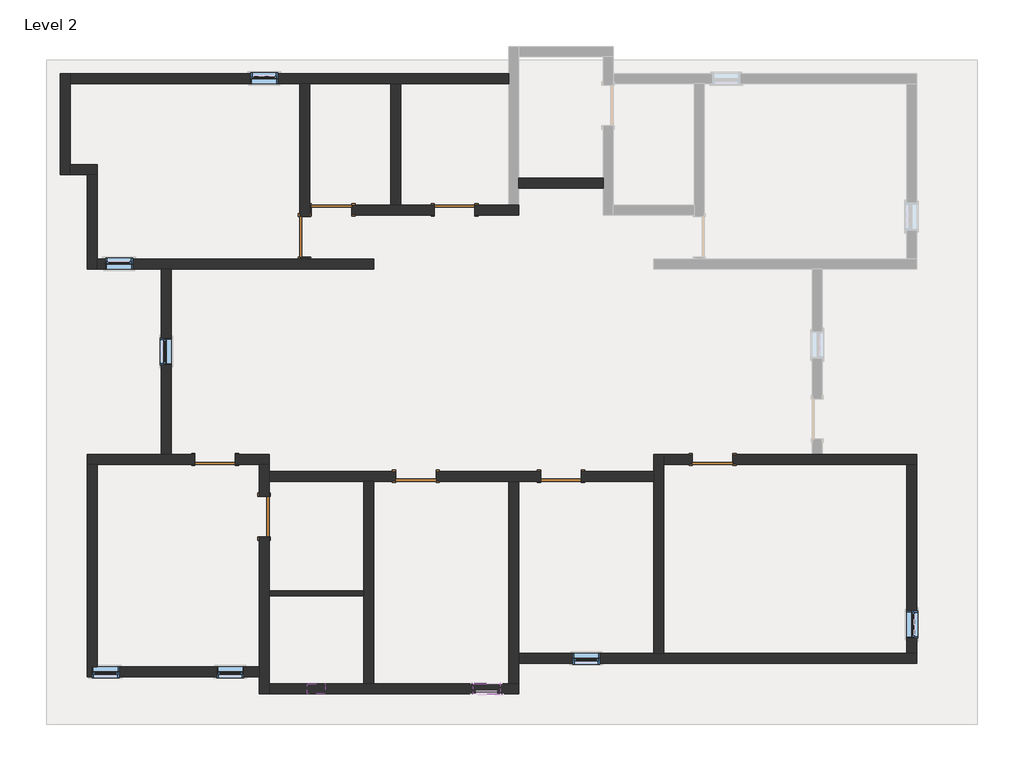
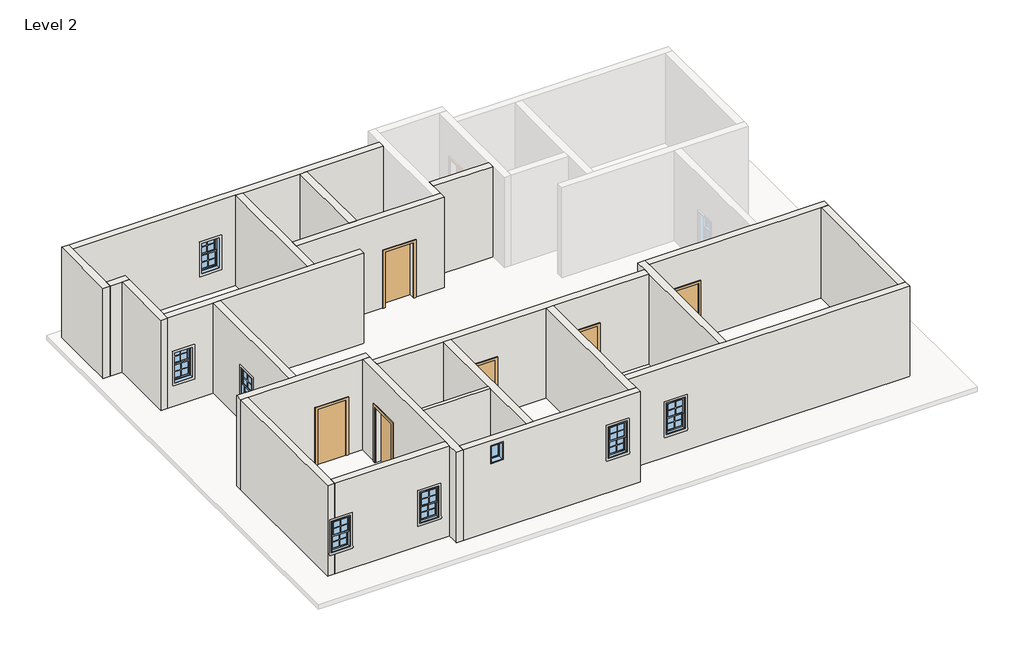
# One storey, part 1 of 2: 23 walls, 9 windows, 8 doors.
"""IFC4 building model written with IfcOpenShell, lengths in millimetres."""

from ifc_helpers import new_model, si_unit, frame, origin, place, context, project, spatial, polyline, outline, extrude, faceted_brep, transform, mapped, element, save
from components import door_89fc3733, door_ef0d591a, window_aa618e30, window_d92165b9

model = new_model("IFC4")

# Units and contexts
model_context = context("Model", 3, world=origin())
ifc_project = project(units=[si_unit("LENGTHUNIT", "METRE", prefix="MILLI")], contexts=[model_context])

# Site, building, storey
site = spatial("IfcSite", under=ifc_project)
building = spatial("IfcBuilding", under=site)
storey = spatial("IfcBuildingStorey", under=building, Name="Level 2", Elevation=3200.4)

# Doors
placement = place(None, origin())
door_shape = door_89fc3733(model_context)
element("IfcDoor", 1, ObjectType="Single-Flush : 36\" x 80\"", at=placement, inside=storey, context=model_context, shape_type="MappedRepresentation", body=[
    mapped(door_shape, transform((-6055.8415084, -1138.2064015, 3200.4), x_axis=(-1.0, 0.0, 0.0), y_axis=(0.0, -1.0, 0.0), z_axis=(0.0, 0.0, 1.0))),
])
element("IfcDoor", 2, ObjectType="Single-Flush : 36\" x 80\"", at=placement, inside=storey, context=model_context, shape_type="MappedRepresentation", body=[
    mapped(door_shape, transform((649.7584916, -757.2064015, 3200.4), x_axis=(-1.0, 0.0, 0.0), y_axis=(0.0, -1.0, 0.0), z_axis=(0.0, 0.0, 1.0))),
])
element("IfcDoor", 3, ObjectType="Single-Flush : 36\" x 80\"", at=placement, inside=storey, context=model_context, shape_type="MappedRepresentation", body=[
    mapped(door_shape, transform((-5179.5415084, 4881.5935985, 3200.4), x_axis=(1.0, 0.0, 0.0), y_axis=(0.0, 1.0, 0.0), z_axis=(0.0, 0.0, 1.0))),
])
element("IfcDoor", 4, ObjectType="Single-Flush : 36\" x 80\"", at=placement, inside=storey, context=model_context, shape_type="MappedRepresentation", body=[
    mapped(door_shape, transform((-2779.2415084, -1138.2064015, 3200.4), x_axis=(-1.0, 0.0, 0.0), y_axis=(0.0, -1.0, 0.0), z_axis=(0.0, 0.0, 1.0))),
])
door_2_shape = door_ef0d591a(model_context)
element("IfcDoor", 5, ObjectType="Single-Flush : 36\" x 80\"", at=placement, inside=storey, context=model_context, shape_type="MappedRepresentation", body=[
    mapped(door_2_shape, transform((-8570.4415084, 4271.9935985, 3200.4), x_axis=(0.0, -1.0, 0.0), y_axis=(1.0, 0.0, 0.0), z_axis=(0.0, 0.0, 1.0))),
])
element("IfcDoor", 6, ObjectType="Single-Flush : 36\" x 80\"", at=placement, inside=storey, context=model_context, shape_type="MappedRepresentation", body=[
    mapped(door_2_shape, transform((-7960.8415084, 4881.5935985, 3200.4), x_axis=(-1.0, 0.0, 0.0), y_axis=(0.0, -1.0, 0.0), z_axis=(0.0, 0.0, 1.0))),
])
element("IfcDoor", 7, ObjectType="Single-Flush : 36\" x 80\"", at=placement, inside=storey, context=model_context, shape_type="MappedRepresentation", body=[
    mapped(door_2_shape, transform((-9484.8415084, -2052.6064015, 3200.4), x_axis=(0.0, 1.0, 0.0), y_axis=(-1.0, 0.0, 0.0), z_axis=(0.0, 0.0, 1.0))),
])
element("IfcDoor", 8, ObjectType="Single-Flush : 36\" x 80\"", at=placement, inside=storey, context=model_context, shape_type="MappedRepresentation", body=[
    mapped(door_2_shape, transform((-10589.7415084, -757.2064015, 3200.4), x_axis=(1.0, 0.0, 0.0), y_axis=(0.0, 1.0, 0.0), z_axis=(0.0, 0.0, 1.0))),
])

# Walls
element("IfcWall", 9, ObjectType="4.5\"", at=placement, inside=storey, context=model_context, shape_type="SweptSolid", body=[
    extrude(outline(polyline([(-7236.9415084, -3843.3848078), (-9370.5415084, -3843.3848078), (-9370.5415084, -3729.0848078), (-7236.9415084, -3729.0848078), (-7236.9415084, -3843.3848078)])), frame((0.0, 0.0, 3200.4), z_axis=(0.0, 0.0, 1.0), x_axis=(1.0, 0.0, 0.0)), (0.0, 0.0, 1.0), 3200.4),
])
element("IfcWall", 10, ObjectType="9\"", at=placement, inside=storey, context=model_context, shape_type="Brep", body=[
    faceted_brep([(-14094.9415084, 7967.6935985, 3200.4), (-14094.9415084, 5681.6935985, 3200.4), (-14094.9415084, 5681.6935985, 6400.8), (-14094.9415084, 7967.6935985, 6400.8), (-13866.3415084, 7967.6935985, 3200.4), (-13866.3415084, 7967.6935985, 6400.8), (-13866.3415084, 7739.0935985, 6400.8), (-13866.3415084, 5910.2935985, 6400.8), (-13866.3415084, 5681.6935985, 6400.8), (-13866.3415084, 5681.6935985, 3200.4), (-13866.3415084, 5910.2935985, 3200.4), (-13866.3415084, 7739.0935985, 3200.4)], [[[0, 1, 2, 3]], [[4, 5, 6, 7, 8, 9, 10, 11]], [[1, 0, 4, 11, 10, 9]], [[3, 2, 8, 7, 6, 5]], [[2, 1, 9, 8]], [[0, 3, 5, 4]]]),
])
element("IfcWall", 11, ObjectType="9\"", at=placement, inside=storey, context=model_context, shape_type="Brep", body=[
    faceted_brep([(-13866.3415084, 5681.6935985, 3200.4), (-13485.3415084, 5681.6935985, 3200.4), (-13256.7415084, 5681.6935985, 3200.4), (-13256.7415084, 5681.6935985, 6400.8), (-13485.3415084, 5681.6935985, 6400.8), (-13866.3415084, 5681.6935985, 6400.8), (-13866.3415084, 5910.2935985, 3200.4), (-13866.3415084, 5910.2935985, 6400.8), (-13256.7415084, 5910.2935985, 6400.8), (-13256.7415084, 5910.2935985, 3200.4)], [[[0, 1, 2, 3, 4, 5]], [[6, 7, 8, 9]], [[2, 1, 0, 6, 9]], [[5, 4, 3, 8, 7]], [[0, 5, 7, 6]], [[3, 2, 9, 8]]]),
])
element("IfcWall", 12, ObjectType="9\"", at=placement, inside=storey, context=model_context, shape_type="Brep", body=[
    faceted_brep([(-13485.3415084, 5681.6935985, 3200.4), (-13485.3415084, 3548.0935985, 3200.4), (-13485.3415084, 3548.0935985, 6400.8), (-13485.3415084, 5681.6935985, 6400.8), (-13256.7415084, 5681.6935985, 3200.4), (-13256.7415084, 5681.6935985, 6400.8), (-13256.7415084, 3776.6935985, 6400.8), (-13256.7415084, 3548.0935985, 6400.8), (-13256.7415084, 3548.0935985, 3200.4), (-13256.7415084, 3776.6935985, 3200.4)], [[[0, 1, 2, 3]], [[4, 5, 6, 7, 8, 9]], [[1, 0, 4, 9, 8]], [[3, 2, 7, 6, 5]], [[0, 3, 5, 4]], [[2, 1, 8, 7]]]),
])
element("IfcWall", 13, ObjectType="9\"", at=placement, inside=storey, context=model_context, shape_type="Brep", body=[
    faceted_brep([(-13256.7415084, 3548.0935985, 3200.4), (-11808.9415084, 3548.0935985, 3200.4), (-11580.3415084, 3548.0935985, 3200.4), (-7008.3415084, 3548.0935985, 3200.4), (-7008.3415084, 3548.0935985, 6400.8), (-11580.3415084, 3548.0935985, 6400.8), (-11808.9415084, 3548.0935985, 6400.8), (-13256.7415084, 3548.0935985, 6400.8), (-13066.2415084, 3548.0935985, 5181.6), (-12456.6415084, 3548.0935985, 5181.6), (-12456.6415084, 3548.0935985, 4114.8), (-13066.2415084, 3548.0935985, 4114.8), (-13256.7415084, 3776.6935985, 3200.4), (-13256.7415084, 3776.6935985, 6400.8), (-8684.7415084, 3776.6935985, 6400.8), (-8456.1415084, 3776.6935985, 6400.8), (-7008.3415084, 3776.6935985, 6400.8), (-7008.3415084, 3776.6935985, 3200.4), (-8456.1415084, 3776.6935985, 3200.4), (-8684.7415084, 3776.6935985, 3200.4), (-13066.2415084, 3776.6935985, 5181.6), (-13066.2415084, 3776.6935985, 4114.8), (-12456.6415084, 3776.6935985, 4114.8), (-12456.6415084, 3776.6935985, 5181.6)], [[[0, 1, 2, 3, 4, 5, 6, 7], [8, 9, 10, 11]], [[12, 13, 14, 15, 16, 17, 18, 19], [20, 21, 22, 23]], [[3, 2, 1, 0, 12, 19, 18, 17]], [[4, 3, 17, 16]], [[7, 6, 5, 4, 16, 15, 14, 13]], [[0, 7, 13, 12]], [[21, 20, 8, 11]], [[22, 21, 11, 10]], [[23, 22, 10, 9]], [[20, 23, 9, 8]]]),
])
element("IfcWall", 14, ObjectType="9\"", at=placement, inside=storey, context=model_context, shape_type="Brep", body=[
    faceted_brep([(-8684.7415084, 3814.7935985, 5232.4), (-8684.7415084, 3814.7935985, 3200.4), (-8684.7415084, 3776.6935985, 3200.4), (-8684.7415084, 3776.6935985, 6400.8), (-8684.7415084, 7739.0935985, 6400.8), (-8684.7415084, 7739.0935985, 3200.4), (-8684.7415084, 4729.1935985, 3200.4), (-8684.7415084, 4729.1935985, 5232.4), (-8456.1415084, 3776.6935985, 3200.4), (-8456.1415084, 3814.7935985, 3200.4), (-8456.1415084, 3814.7935985, 5232.4), (-8456.1415084, 4729.1935985, 5232.4), (-8456.1415084, 4729.1935985, 3200.4), (-8456.1415084, 4767.2935985, 3200.4), (-8456.1415084, 4995.8935985, 3200.4), (-8456.1415084, 7739.0935985, 3200.4), (-8456.1415084, 7739.0935985, 6400.8), (-8456.1415084, 4995.8935985, 6400.8), (-8456.1415084, 4767.2935985, 6400.8), (-8456.1415084, 3776.6935985, 6400.8)], [[[0, 1, 2, 3, 4, 5, 6, 7]], [[8, 9, 10, 11, 12, 13, 14, 15, 16, 17, 18, 19]], [[6, 5, 15, 14, 13, 12]], [[2, 1, 9, 8]], [[4, 3, 19, 18, 17, 16]], [[3, 2, 8, 19]], [[5, 4, 16, 15]], [[10, 9, 1, 0]], [[11, 10, 0, 7]], [[12, 11, 7, 6]]]),
])
element("IfcWall", 15, ObjectType="9\"", at=placement, inside=storey, context=model_context, shape_type="Brep", body=[
    faceted_brep([(-3960.3415084, 7967.6935985, 3200.4), (-13866.3415084, 7967.6935985, 3200.4), (-13866.3415084, 7967.6935985, 6400.8), (-3960.3415084, 7967.6935985, 6400.8), (-9789.6415084, 7967.6935985, 5181.6), (-9789.6415084, 7967.6935985, 4114.8), (-9180.0415084, 7967.6935985, 4114.8), (-9180.0415084, 7967.6935985, 5181.6), (-3960.3415084, 7739.0935985, 3200.4), (-3960.3415084, 7739.0935985, 6400.8), (-6398.7415084, 7739.0935985, 6400.8), (-6627.3415084, 7739.0935985, 6400.8), (-8456.1415084, 7739.0935985, 6400.8), (-8684.7415084, 7739.0935985, 6400.8), (-13866.3415084, 7739.0935985, 6400.8), (-13866.3415084, 7739.0935985, 3200.4), (-8684.7415084, 7739.0935985, 3200.4), (-8456.1415084, 7739.0935985, 3200.4), (-6627.3415084, 7739.0935985, 3200.4), (-6398.7415084, 7739.0935985, 3200.4), (-9789.6415084, 7739.0935985, 5181.6), (-9180.0415084, 7739.0935985, 5181.6), (-9180.0415084, 7739.0935985, 4114.8), (-9789.6415084, 7739.0935985, 4114.8)], [[[0, 1, 2, 3], [4, 5, 6, 7]], [[8, 9, 10, 11, 12, 13, 14, 15, 16, 17, 18, 19], [20, 21, 22, 23]], [[1, 0, 8, 19, 18, 17, 16, 15]], [[3, 2, 14, 13, 12, 11, 10, 9]], [[2, 1, 15, 14]], [[0, 3, 9, 8]], [[5, 4, 20, 23]], [[6, 5, 23, 22]], [[7, 6, 22, 21]], [[4, 7, 21, 20]]]),
])
element("IfcWall", 16, ObjectType="9\"", at=placement, inside=storey, context=model_context, shape_type="Brep", body=[
    faceted_brep([(-3731.7415084, 4995.8935985, 3200.4), (-3960.3415084, 4995.8935985, 3200.4), (-4722.3415084, 4995.8935985, 3200.4), (-4722.3415084, 4995.8935985, 5232.4), (-5636.7415084, 4995.8935985, 5232.4), (-5636.7415084, 4995.8935985, 3200.4), (-6398.7415084, 4995.8935985, 3200.4), (-6627.3415084, 4995.8935985, 3200.4), (-7503.6415084, 4995.8935985, 3200.4), (-7503.6415084, 4995.8935985, 5232.4), (-8418.0415084, 4995.8935985, 5232.4), (-8418.0415084, 4995.8935985, 3200.4), (-8456.1415084, 4995.8935985, 3200.4), (-8456.1415084, 4995.8935985, 6400.8), (-6627.3415084, 4995.8935985, 6400.8), (-6398.7415084, 4995.8935985, 6400.8), (-3960.3415084, 4995.8935985, 6400.8), (-3731.7415084, 4995.8935985, 6400.8), (-4722.3415084, 4767.2935985, 5232.4), (-4722.3415084, 4767.2935985, 3200.4), (-3731.7415084, 4767.2935985, 3200.4), (-3731.7415084, 4767.2935985, 6400.8), (-8456.1415084, 4767.2935985, 6400.8), (-8456.1415084, 4767.2935985, 3200.4), (-8418.0415084, 4767.2935985, 3200.4), (-8418.0415084, 4767.2935985, 5232.4), (-7503.6415084, 4767.2935985, 5232.4), (-7503.6415084, 4767.2935985, 3200.4), (-5636.7415084, 4767.2935985, 3200.4), (-5636.7415084, 4767.2935985, 5232.4)], [[[0, 1, 2, 3, 4, 5, 6, 7, 8, 9, 10, 11, 12, 13, 14, 15, 16, 17]], [[18, 19, 20, 21, 22, 23, 24, 25, 26, 27, 28, 29]], [[12, 11, 24, 23]], [[28, 27, 8, 7, 6, 5]], [[20, 19, 2, 1, 0]], [[17, 16, 15, 14, 13, 22, 21]], [[13, 12, 23, 22]], [[0, 17, 21, 20]], [[25, 24, 11, 10]], [[26, 25, 10, 9]], [[27, 26, 9, 8]], [[3, 2, 19, 18]], [[4, 3, 18, 29]], [[5, 4, 29, 28]]]),
])
element("IfcWall", 17, ObjectType="9\"", at=placement, inside=storey, context=model_context, shape_type="SweptSolid", body=[
    extrude(outline(polyline([(-6627.3415084, 4995.8935985), (-6627.3415084, 7739.0935985), (-6398.7415084, 7739.0935985), (-6398.7415084, 4995.8935985), (-6627.3415084, 4995.8935985)])), frame((0.0, 0.0, 3200.4), z_axis=(0.0, 0.0, 1.0), x_axis=(1.0, 0.0, 0.0)), (0.0, 0.0, 1.0), 3200.4),
])
element("IfcWall", 18, ObjectType="9\"", at=placement, inside=storey, context=model_context, shape_type="SweptSolid", body=[
    extrude(outline(polyline([(-3731.7415084, 5605.4935985), (-1826.7415084, 5605.4935985), (-1826.7415084, 5376.8935985), (-3731.7415084, 5376.8935985), (-3731.7415084, 5605.4935985)])), frame((0.0, 0.0, 3200.4), z_axis=(0.0, 0.0, 1.0), x_axis=(1.0, 0.0, 0.0)), (0.0, 0.0, 1.0), 3200.4),
])
element("IfcWall", 19, ObjectType="9\"", at=placement, inside=storey, context=model_context, shape_type="SweptSolid", body=[
    extrude(outline(polyline([(3548.0935985, 3200.4), (-642.9064015, 3200.4), (-642.9064015, 6400.8), (3548.0935985, 6400.8), (3548.0935985, 3200.4)]), holes=[polyline([(1376.3935985, 5181.6), (1376.3935985, 4114.8), (1985.9935985, 4114.8), (1985.9935985, 5181.6), (1376.3935985, 5181.6)])]), frame((-11808.9415084, 0.0, 0.0), z_axis=(1.0, 0.0, 0.0), x_axis=(0.0, 1.0, 0.0)), (0.0, 0.0, 1.0), 228.6),
])
element("IfcWall", 20, ObjectType="9\"", at=placement, inside=storey, context=model_context, shape_type="Brep", body=[
    faceted_brep([(-9370.5415084, -642.9064015, 3200.4), (-10132.5415084, -642.9064015, 3200.4), (-10132.5415084, -642.9064015, 5232.4), (-11046.9415084, -642.9064015, 5232.4), (-11046.9415084, -642.9064015, 3200.4), (-11580.3415084, -642.9064015, 3200.4), (-11808.9415084, -642.9064015, 3200.4), (-13485.3415084, -642.9064015, 3200.4), (-13485.3415084, -642.9064015, 6400.8), (-11808.9415084, -642.9064015, 6400.8), (-11580.3415084, -642.9064015, 6400.8), (-9370.5415084, -642.9064015, 6400.8), (-10132.5415084, -871.5064015, 5232.4), (-10132.5415084, -871.5064015, 3200.4), (-9599.1415084, -871.5064015, 3200.4), (-9370.5415084, -871.5064015, 3200.4), (-9370.5415084, -871.5064015, 6400.8), (-9599.1415084, -871.5064015, 6400.8), (-13256.7415084, -871.5064015, 6400.8), (-13485.3415084, -871.5064015, 6400.8), (-13485.3415084, -871.5064015, 3200.4), (-13256.7415084, -871.5064015, 3200.4), (-11046.9415084, -871.5064015, 3200.4), (-11046.9415084, -871.5064015, 5232.4)], [[[0, 1, 2, 3, 4, 5, 6, 7, 8, 9, 10, 11]], [[12, 13, 14, 15, 16, 17, 18, 19, 20, 21, 22, 23]], [[15, 14, 13, 1, 0]], [[22, 21, 20, 7, 6, 5, 4]], [[11, 10, 9, 8, 19, 18, 17, 16]], [[8, 7, 20, 19]], [[0, 11, 16, 15]], [[2, 1, 13, 12]], [[3, 2, 12, 23]], [[4, 3, 23, 22]]]),
])
element("IfcWall", 21, ObjectType="9\"", at=placement, inside=storey, context=model_context, shape_type="Brep", body=[
    faceted_brep([(-13485.3415084, -871.5064015, 3200.4), (-13485.3415084, -5672.1064015, 3200.4), (-13485.3415084, -5672.1064015, 6400.8), (-13485.3415084, -871.5064015, 6400.8), (-13256.7415084, -5672.1064015, 3200.4), (-13256.7415084, -5443.5064015, 3200.4), (-13256.7415084, -871.5064015, 3200.4), (-13256.7415084, -871.5064015, 6400.8), (-13256.7415084, -5443.5064015, 6400.8), (-13256.7415084, -5672.1064015, 6400.8), (-13256.7415084, -5672.1064015, 5181.6), (-13256.7415084, -5443.5064015, 5181.6), (-13256.7415084, -5443.5064015, 4114.8), (-13256.7415084, -5672.1064015, 4114.8), (-13371.0415084, -5672.1064015, 4114.8), (-13371.0415084, -5672.1064015, 5181.6), (-13371.0415084, -5443.5064015, 5181.6), (-13371.0415084, -5443.5064015, 4114.8)], [[[0, 1, 2, 3]], [[4, 5, 6, 7, 8, 9, 10, 11, 12, 13]], [[1, 0, 6, 5, 4]], [[3, 2, 9, 8, 7]], [[0, 3, 7, 6]], [[2, 1, 4, 13, 14, 15, 10, 9]], [[16, 17, 12, 11]], [[17, 14, 13, 12]], [[17, 16, 15, 14]], [[15, 16, 11, 10]]]),
])
element("IfcWall", 22, ObjectType="9\"", at=placement, inside=storey, context=model_context, shape_type="SweptSolid", body=[
    extrude(outline(polyline([(3200.4, -13256.7415084), (3200.4, -9599.1415084), (6400.8, -9599.1415084), (6400.8, -13256.7415084), (5181.6, -13256.7415084), (5181.6, -12761.4415084), (4114.8, -12761.4415084), (4114.8, -13256.7415084), (3200.4, -13256.7415084)]), holes=[polyline([(5181.6, -9942.0415084), (4114.8, -9942.0415084), (4114.8, -10551.6415084), (5181.6, -10551.6415084), (5181.6, -9942.0415084)])]), frame((0.0, -5672.1064015, 0.0), z_axis=(0.0, 1.0, 0.0), x_axis=(0.0, 0.0, 1.0)), (0.0, 0.0, 1.0), 228.6),
])
element("IfcWall", 23, ObjectType="9\"", at=placement, inside=storey, context=model_context, shape_type="Brep", body=[
    faceted_brep([(-9599.1415084, -871.5064015, 3200.4), (-9599.1415084, -1595.4064015, 3200.4), (-9599.1415084, -1595.4064015, 5232.4), (-9599.1415084, -2509.8064015, 5232.4), (-9599.1415084, -2509.8064015, 3200.4), (-9599.1415084, -5443.5064015, 3200.4), (-9599.1415084, -5672.1064015, 3200.4), (-9599.1415084, -6053.1848078, 3200.4), (-9599.1415084, -6053.1848078, 6400.8), (-9599.1415084, -5672.1064015, 6400.8), (-9599.1415084, -5443.5064015, 6400.8), (-9599.1415084, -871.5064015, 6400.8), (-9370.5415084, -1595.4064015, 5232.4), (-9370.5415084, -1595.4064015, 3200.4), (-9370.5415084, -1252.5064015, 3200.4), (-9370.5415084, -1023.9064015, 3200.4), (-9370.5415084, -871.5064015, 3200.4), (-9370.5415084, -871.5064015, 6400.8), (-9370.5415084, -1023.9064015, 6400.8), (-9370.5415084, -1252.5064015, 6400.8), (-9370.5415084, -3729.0848078, 6400.8), (-9370.5415084, -3843.3848078, 6400.8), (-9370.5415084, -5824.5848078, 6400.8), (-9370.5415084, -6053.1848078, 6400.8), (-9370.5415084, -6053.1848078, 3200.4), (-9370.5415084, -5824.5848078, 3200.4), (-9370.5415084, -3843.3848078, 3200.4), (-9370.5415084, -3729.0848078, 3200.4), (-9370.5415084, -2509.8064015, 3200.4), (-9370.5415084, -2509.8064015, 5232.4)], [[[0, 1, 2, 3, 4, 5, 6, 7, 8, 9, 10, 11]], [[12, 13, 14, 15, 16, 17, 18, 19, 20, 21, 22, 23, 24, 25, 26, 27, 28, 29]], [[28, 27, 26, 25, 24, 7, 6, 5, 4]], [[16, 15, 14, 13, 1, 0]], [[11, 10, 9, 8, 23, 22, 21, 20, 19, 18, 17]], [[0, 11, 17, 16]], [[8, 7, 24, 23]], [[2, 1, 13, 12]], [[3, 2, 12, 29]], [[4, 3, 29, 28]]]),
])
element("IfcWall", 24, ObjectType="9\"", at=placement, inside=storey, context=model_context, shape_type="Brep", body=[
    faceted_brep([(-3731.7415084, -5824.5848078, 3200.4), (-3960.3415084, -5824.5848078, 3200.4), (-7008.3415084, -5824.5848078, 3200.4), (-7236.9415084, -5824.5848078, 3200.4), (-9370.5415084, -5824.5848078, 3200.4), (-9370.5415084, -5824.5848078, 6400.8), (-7236.9415084, -5824.5848078, 6400.8), (-7008.3415084, -5824.5848078, 6400.8), (-3960.3415084, -5824.5848078, 6400.8), (-3731.7415084, -5824.5848078, 6400.8), (-8100.5415084, -5824.5848078, 6248.4), (-8506.9415084, -5824.5848078, 6248.4), (-8506.9415084, -5824.5848078, 5638.8), (-8100.5415084, -5824.5848078, 5638.8), (-4150.8415084, -5824.5848078, 5585.3887433), (-4760.4415084, -5824.5848078, 5585.3887433), (-4760.4415084, -5824.5848078, 4518.5887433), (-4150.8415084, -5824.5848078, 4518.5887433), (-3731.7415084, -6053.1848078, 3200.4), (-3731.7415084, -6053.1848078, 6400.8), (-9370.5415084, -6053.1848078, 6400.8), (-9370.5415084, -6053.1848078, 3200.4), (-8100.5415084, -6053.1848078, 6248.4), (-8100.5415084, -6053.1848078, 5638.8), (-8506.9415084, -6053.1848078, 5638.8), (-8506.9415084, -6053.1848078, 6248.4), (-4150.8415084, -6053.1848078, 5585.3887433), (-4150.8415084, -6053.1848078, 4518.5887433), (-4760.4415084, -6053.1848078, 4518.5887433), (-4760.4415084, -6053.1848078, 5585.3887433)], [[[0, 1, 2, 3, 4, 5, 6, 7, 8, 9], [10, 11, 12, 13], [14, 15, 16, 17]], [[18, 19, 20, 21], [22, 23, 24, 25], [26, 27, 28, 29]], [[4, 3, 2, 1, 0, 18, 21]], [[9, 8, 7, 6, 5, 20, 19]], [[5, 4, 21, 20]], [[0, 9, 19, 18]], [[23, 22, 10, 13]], [[24, 23, 13, 12]], [[25, 24, 12, 11]], [[22, 25, 11, 10]], [[27, 26, 14, 17]], [[28, 27, 17, 16]], [[29, 28, 16, 15]], [[26, 29, 15, 14]]]),
])
element("IfcWall", 25, ObjectType="9\"", at=placement, inside=storey, context=model_context, shape_type="Brep", body=[
    faceted_brep([(-7008.3415084, -5824.5848078, 3200.4), (-7008.3415084, -1252.5064015, 3200.4), (-7008.3415084, -1252.5064015, 6400.8), (-7008.3415084, -5824.5848078, 6400.8), (-7236.9415084, -5824.5848078, 3200.4), (-7236.9415084, -5824.5848078, 6400.8), (-7236.9415084, -3843.3848078, 6400.8), (-7236.9415084, -3729.0848078, 6400.8), (-7236.9415084, -1252.5064015, 6400.8), (-7236.9415084, -1252.5064015, 3200.4), (-7236.9415084, -3729.0848078, 3200.4), (-7236.9415084, -3843.3848078, 3200.4)], [[[0, 1, 2, 3]], [[4, 5, 6, 7, 8, 9, 10, 11]], [[1, 0, 4, 11, 10, 9]], [[3, 2, 8, 7, 6, 5]], [[0, 3, 5, 4]], [[2, 1, 9, 8]]]),
])
element("IfcWall", 26, ObjectType="9\"", at=placement, inside=storey, context=model_context, shape_type="Brep", body=[
    faceted_brep([(-3960.3415084, -1252.5064015, 3200.4), (-3960.3415084, -5824.5848078, 3200.4), (-3960.3415084, -5824.5848078, 6400.8), (-3960.3415084, -1252.5064015, 6400.8), (-3731.7415084, -1252.5064015, 3200.4), (-3731.7415084, -1252.5064015, 6400.8), (-3731.7415084, -5138.7064015, 6400.8), (-3731.7415084, -5367.3064015, 6400.8), (-3731.7415084, -5824.5848078, 6400.8), (-3731.7415084, -5824.5848078, 3200.4), (-3731.7415084, -5367.3064015, 3200.4), (-3731.7415084, -5138.7064015, 3200.4)], [[[0, 1, 2, 3]], [[4, 5, 6, 7, 8, 9, 10, 11]], [[1, 0, 4, 11, 10, 9]], [[3, 2, 8, 7, 6, 5]], [[2, 1, 9, 8]], [[0, 3, 5, 4]]]),
])
element("IfcWall", 27, ObjectType="9\"", at=placement, inside=storey, context=model_context, shape_type="Brep", body=[
    faceted_brep([(-3236.4415084, -1023.9064015, 5232.4), (-3236.4415084, -1023.9064015, 3200.4), (-5598.6415084, -1023.9064015, 3200.4), (-5598.6415084, -1023.9064015, 5232.4), (-6513.0415084, -1023.9064015, 5232.4), (-6513.0415084, -1023.9064015, 3200.4), (-9370.5415084, -1023.9064015, 3200.4), (-9370.5415084, -1023.9064015, 6400.8), (-683.7415084, -1023.9064015, 6400.8), (-683.7415084, -1023.9064015, 3200.4), (-2322.0415084, -1023.9064015, 3200.4), (-2322.0415084, -1023.9064015, 5232.4), (-5598.6415084, -1252.5064015, 3200.4), (-3960.3415084, -1252.5064015, 3200.4), (-3731.7415084, -1252.5064015, 3200.4), (-3236.4415084, -1252.5064015, 3200.4), (-3236.4415084, -1252.5064015, 5232.4), (-2322.0415084, -1252.5064015, 5232.4), (-2322.0415084, -1252.5064015, 3200.4), (-683.7415084, -1252.5064015, 3200.4), (-683.7415084, -1252.5064015, 6400.8), (-3731.7415084, -1252.5064015, 6400.8), (-3960.3415084, -1252.5064015, 6400.8), (-7008.3415084, -1252.5064015, 6400.8), (-7236.9415084, -1252.5064015, 6400.8), (-9370.5415084, -1252.5064015, 6400.8), (-9370.5415084, -1252.5064015, 3200.4), (-7236.9415084, -1252.5064015, 3200.4), (-7008.3415084, -1252.5064015, 3200.4), (-6513.0415084, -1252.5064015, 3200.4), (-6513.0415084, -1252.5064015, 5232.4), (-5598.6415084, -1252.5064015, 5232.4)], [[[0, 1, 2, 3, 4, 5, 6, 7, 8, 9, 10, 11]], [[12, 13, 14, 15, 16, 17, 18, 19, 20, 21, 22, 23, 24, 25, 26, 27, 28, 29, 30, 31]], [[6, 5, 29, 28, 27, 26]], [[10, 9, 19, 18]], [[2, 1, 15, 14, 13, 12]], [[8, 7, 25, 24, 23, 22, 21, 20]], [[7, 6, 26, 25]], [[9, 8, 20, 19]], [[30, 29, 5, 4]], [[31, 30, 4, 3]], [[12, 31, 3, 2]], [[16, 15, 1, 0]], [[17, 16, 0, 11]], [[18, 17, 11, 10]]]),
])
element("IfcWall", 28, ObjectType="9\"", at=placement, inside=storey, context=model_context, shape_type="Brep", body=[
    faceted_brep([(5259.8584916, -5138.7064015, 3200.4), (5031.2584916, -5138.7064015, 3200.4), (-455.1415084, -5138.7064015, 3200.4), (-683.7415084, -5138.7064015, 3200.4), (-3731.7415084, -5138.7064015, 3200.4), (-3731.7415084, -5138.7064015, 6400.8), (-683.7415084, -5138.7064015, 6400.8), (-455.1415084, -5138.7064015, 6400.8), (5031.2584916, -5138.7064015, 6400.8), (5259.8584916, -5138.7064015, 6400.8), (-1902.9415084, -5138.7064015, 5181.6), (-2512.5415084, -5138.7064015, 5181.6), (-2512.5415084, -5138.7064015, 4114.8), (-1902.9415084, -5138.7064015, 4114.8), (5259.8584916, -5367.3064015, 3200.4), (5259.8584916, -5367.3064015, 6400.8), (-3731.7415084, -5367.3064015, 6400.8), (-3731.7415084, -5367.3064015, 3200.4), (-1902.9415084, -5367.3064015, 5181.6), (-1902.9415084, -5367.3064015, 4114.8), (-2512.5415084, -5367.3064015, 4114.8), (-2512.5415084, -5367.3064015, 5181.6)], [[[0, 1, 2, 3, 4, 5, 6, 7, 8, 9], [10, 11, 12, 13]], [[14, 15, 16, 17], [18, 19, 20, 21]], [[4, 3, 2, 1, 0, 14, 17]], [[9, 8, 7, 6, 5, 16, 15]], [[5, 4, 17, 16]], [[0, 9, 15, 14]], [[19, 18, 10, 13]], [[20, 19, 13, 12]], [[21, 20, 12, 11]], [[18, 21, 11, 10]]]),
])
element("IfcWall", 29, ObjectType="9\"", at=placement, inside=storey, context=model_context, shape_type="Brep", body=[
    faceted_brep([(-683.7415084, -642.9064015, 3200.4), (-683.7415084, -1023.9064015, 3200.4), (-683.7415084, -1252.5064015, 3200.4), (-683.7415084, -5138.7064015, 3200.4), (-683.7415084, -5138.7064015, 6400.8), (-683.7415084, -1252.5064015, 6400.8), (-683.7415084, -1023.9064015, 6400.8), (-683.7415084, -642.9064015, 6400.8), (-455.1415084, -642.9064015, 3200.4), (-455.1415084, -642.9064015, 6400.8), (-455.1415084, -871.5064015, 6400.8), (-455.1415084, -5138.7064015, 6400.8), (-455.1415084, -5138.7064015, 3200.4), (-455.1415084, -871.5064015, 3200.4)], [[[0, 1, 2, 3, 4, 5, 6, 7]], [[8, 9, 10, 11, 12, 13]], [[3, 2, 1, 0, 8, 13, 12]], [[7, 6, 5, 4, 11, 10, 9]], [[4, 3, 12, 11]], [[0, 7, 9, 8]]]),
])
element("IfcWall", 30, ObjectType="9\"", at=placement, inside=storey, context=model_context, shape_type="Brep", body=[
    faceted_brep([(192.5584916, -642.9064015, 5232.4), (192.5584916, -642.9064015, 3200.4), (-455.1415084, -642.9064015, 3200.4), (-455.1415084, -642.9064015, 6400.8), (2897.6584916, -642.9064015, 6400.8), (3126.2584916, -642.9064015, 6400.8), (5259.8584916, -642.9064015, 6400.8), (5259.8584916, -642.9064015, 3200.4), (3126.2584916, -642.9064015, 3200.4), (2897.6584916, -642.9064015, 3200.4), (1106.9584916, -642.9064015, 3200.4), (1106.9584916, -642.9064015, 5232.4), (-455.1415084, -871.5064015, 3200.4), (192.5584916, -871.5064015, 3200.4), (192.5584916, -871.5064015, 5232.4), (1106.9584916, -871.5064015, 5232.4), (1106.9584916, -871.5064015, 3200.4), (5031.2584916, -871.5064015, 3200.4), (5259.8584916, -871.5064015, 3200.4), (5259.8584916, -871.5064015, 6400.8), (5031.2584916, -871.5064015, 6400.8), (-455.1415084, -871.5064015, 6400.8)], [[[0, 1, 2, 3, 4, 5, 6, 7, 8, 9, 10, 11]], [[12, 13, 14, 15, 16, 17, 18, 19, 20, 21]], [[2, 1, 13, 12]], [[10, 9, 8, 7, 18, 17, 16]], [[6, 5, 4, 3, 21, 20, 19]], [[3, 2, 12, 21]], [[7, 6, 19, 18]], [[14, 13, 1, 0]], [[15, 14, 0, 11]], [[16, 15, 11, 10]]]),
])
element("IfcWall", 31, ObjectType="9\"", at=placement, inside=storey, context=model_context, shape_type="SweptSolid", body=[
    extrude(outline(polyline([(-871.5064015, 3200.4), (-5138.7064015, 3200.4), (-5138.7064015, 6400.8), (-871.5064015, 6400.8), (-871.5064015, 3200.4)]), holes=[polyline([(-4186.2064015, 5181.6), (-4795.8064015, 5181.6), (-4795.8064015, 4114.8), (-4186.2064015, 4114.8), (-4186.2064015, 5181.6)])]), frame((5031.2584916, 0.0, 0.0), z_axis=(1.0, 0.0, 0.0), x_axis=(0.0, 1.0, 0.0)), (0.0, 0.0, 1.0), 228.6),
])

# Windows
window_shape = window_aa618e30(model_context)
element("IfcWindow", 32, ObjectType="Fixed : 16\" x 24\"", at=placement, inside=storey, context=model_context, shape_type="MappedRepresentation", body=[
    mapped(window_shape, transform((-8265.6415084, -5938.8848078, 4724.4), x_axis=(1.0, 0.0, 0.0), y_axis=(0.0, 1.0, 0.0), z_axis=(0.0, 0.0, 1.0))),
])
window_2_shape = window_d92165b9(model_context)
element("IfcWindow", 33, ObjectType="Window-Double-Hung : 24\" x 42\"", at=placement, inside=storey, context=model_context, shape_type="MappedRepresentation", body=[
    mapped(window_2_shape, transform((-9484.8415084, 7853.3935985, 3200.4), x_axis=(1.0, 0.0, 0.0), y_axis=(0.0, 1.0, 0.0), z_axis=(0.0, 0.0, 1.0))),
])
element("IfcWindow", 34, ObjectType="Window-Double-Hung : 24\" x 42\"", at=placement, inside=storey, context=model_context, shape_type="MappedRepresentation", body=[
    mapped(window_2_shape, transform((-12761.4415084, 3662.3935985, 3200.4), x_axis=(1.0, 0.0, 0.0), y_axis=(0.0, 1.0, 0.0), z_axis=(0.0, 0.0, 1.0))),
])
element("IfcWindow", 35, ObjectType="Window-Double-Hung : 24\" x 42\"", at=placement, inside=storey, context=model_context, shape_type="MappedRepresentation", body=[
    mapped(window_2_shape, transform((-13066.2415084, -5557.8064015, 3200.4), x_axis=(-1.0, 0.0, 0.0), y_axis=(0.0, -1.0, 0.0), z_axis=(0.0, 0.0, 1.0))),
])
element("IfcWindow", 36, ObjectType="Window-Double-Hung : 24\" x 42\"", at=placement, inside=storey, context=model_context, shape_type="MappedRepresentation", body=[
    mapped(window_2_shape, transform((-10246.8415084, -5557.8064015, 3200.4), x_axis=(-1.0, 0.0, 0.0), y_axis=(0.0, -1.0, 0.0), z_axis=(0.0, 0.0, 1.0))),
])
element("IfcWindow", 37, ObjectType="Window-Double-Hung : 24\" x 42\"", at=placement, inside=storey, context=model_context, shape_type="MappedRepresentation", body=[
    mapped(window_2_shape, transform((-11694.6415084, 1681.1935985, 3200.4), x_axis=(0.0, 1.0, 0.0), y_axis=(-1.0, 0.0, 0.0), z_axis=(0.0, 0.0, 1.0))),
])
element("IfcWindow", 38, ObjectType="Window-Double-Hung : 24\" x 42\"", at=placement, inside=storey, context=model_context, shape_type="MappedRepresentation", body=[
    mapped(window_2_shape, transform((-2207.7415084, -5253.0064015, 3200.4), x_axis=(-1.0, 0.0, 0.0), y_axis=(0.0, -1.0, 0.0), z_axis=(0.0, 0.0, 1.0))),
])
element("IfcWindow", 39, ObjectType="Window-Double-Hung : 24\" x 42\"", at=placement, inside=storey, context=model_context, shape_type="MappedRepresentation", body=[
    mapped(window_2_shape, transform((5145.5584916, -4491.0064015, 3200.4), x_axis=(0.0, -1.0, 0.0), y_axis=(1.0, 0.0, 0.0), z_axis=(0.0, 0.0, 1.0))),
])
element("IfcWindow", 40, ObjectType="Window-Double-Hung : 24\" x 42\"", at=placement, inside=storey, context=model_context, shape_type="MappedRepresentation", body=[
    mapped(window_2_shape, transform((-4455.6415084, -5938.8848078, 3604.1887433), x_axis=(-1.0, 0.0, 0.0), y_axis=(0.0, -1.0, 0.0), z_axis=(0.0, 0.0, 1.0))),
])

save(model, "model.ifc")

# Revit data of these elements
# Type "Single-Flush : 36\" x 80\""
#   Type Mark = "6"
#   Construction Type Id = "MDOOR"
#   Assembly Code = "C1020"
#   Analytic Construction = "Metal"
#   Thickness = 0' - 2"
#   Heat Transfer Coefficient (U) = 0.651978 BTU/(h·ft²·°F)
#   Height = 6' - 8"
#   Trim Projection Ext = 0' - 1"
#   Trim Projection Int = 0' - 1"
#   Trim Width = 0' - 3"
#   Width = 3' - 0"
#   Define Thermal Properties by = 1
#   Define Thermal Properties by = 1
#   Door Material = Door - Panel
#   Frame Material = Door - Frame
#   Visual Light Transmittance = 0
#   Solar Heat Gain Coefficient = 0
#   Function = (empty or 0)
#   Wall Closure = (empty or 0)
# Type "4.5\""
#   Assembly Code = "B2010"
#   Layers, outside or top first: 0' - 4 1/2" no material (function 1)
# Type "9\""
#   Assembly Code = "B2010"
#   Layers, outside or top first: 0' - 9" no material (function 1)
# Type "Fixed : 16\" x 24\""
#   Type Mark = "4"
#   Construction Type Id = "GSP4R"
#   Assembly Code = "B2020100"
#   Analytic Construction = "1/8 in Pilkington single glazing"
#   Visual Light Transmittance = 0.9
#   Solar Heat Gain Coefficient = 0.78
#   Heat Transfer Coefficient (U) = 0.6496 BTU/(h·ft²·°F)
#   Height = 2' - 0"
#   Default Sill Height = 3' - 0"
#   Width = 1' - 4"
#   Window Inset = 0' - 0 3/4"
#   Define Thermal Properties by = 1
#   Define Thermal Properties by = 1
#   Glass Pane Material = Glass
#   Sash Material = Sash
#   Wall Closure = (empty or 0)
# Type "Window-Double-Hung : 24\" x 42\""
#   Type Mark = "10"
#   Fire Rating = "0.5h"
#   Construction Type Id = "DG-DR"
#   Assembly Code = "B2020100"
#   Analytic Construction = "Double glazing - domestic"
#   Wall Thickness [instance default] = 0' - 6"
#   Window Inset [instance default] = 0' - 0"
#   Visual Light Transmittance = 0.81
#   Thermal Resistance (R) = 1.8146 (h·ft²·°F)/BTU
#   Solar Heat Gain Coefficient = 0.76
#   Muntin Width = 1' - 6"
#   Muntin Height = 1' - 5 1/8"
#   Interior Wall Closure [instance default] = 0' - 1 1/2"
#   Rough Width = 2' - 0 1/2"
#   Rough Height = 3' - 6 1/2"
#   Frame Extension [instance default] = 0' - 1 1/4"
#   Exterior Wall Closure [instance default] = 0' - 0 1/2"
#   Extension Jamb [instance default] = 0' - 1 1/2"
#   Heat Transfer Coefficient (U) = 0.5511 BTU/(h·ft²·°F)
#   Height = 3' - 6"
#   Width = 2' - 0"
#   Define Thermal Properties by = 1
#   Top Muntin Visibility = yes
#   Indicator Visibility [instance default] = yes
#   Extension Jamb Visibility [instance default] = yes
#   Interior Trim Visibility [instance default] = yes
#   Exterior Trim Visibility [instance default] = yes
#   Define Thermal Properties by = 1
#   Bottom Muntin Visibility = yes
#   Muntin Pattern = Muntin Pattern_2x2 : Muntin Pattern_2x2
#   Interior Trim Material = Wood - Stained
#   Interior Trim = Trim-Window-Interior-Flat : Picture Frame
#   Exterior Trim Material = Clad - White
#   Exterior Trim = Trim-Window-Exterior-Flat : with Sill
#   Glass Panel Material = Glass
#   Exterior Frame Material = Clad - White
#   Interior Frame Material = Wood - Stained
#   Wall Closure = (empty or 0)
# Elements 1, 2, 3, 4, 5, 6, 7, 8 (IfcDoor, "Single-Flush : 36\" x 80\"")
#   Phase Created = New Construction
#   Materials on its faces: "Door - Frame", "Door - Panel"
# Element 9 (IfcWall, "4.5\"")
#   Top Offset = 0' - 0"
#   Base Offset = 0' - 0"
#   wall height = 10' - 6"
#   Phase Created = New Construction
#   Base Constraint = Level 2
#   Top Constraint = Level 3
#   Materials on its faces: "Default Wall"
# Elements 10, 11, 12, 13, 14, 15, 16, 17, 18, 19, 20, 21, 22, 25, 26, 27, 28, 29, 30, 31 (IfcWall, "9\"")
#   Top Offset = 0' - 0"
#   Base Offset = 0' - 0"
#   wall height = 10' - 6"
#   Phase Created = New Construction
#   Base Constraint = Level 2
#   Top Constraint = Level 3
#   Materials on its faces: "Default Wall"
# Elements 23, 24 (IfcWall, "9\"")
#   Top Offset = 0' - 0"
#   Base Offset = 0' - 0"
#   wall height = 10' - 6"
#   Phase Created = New Construction
#   Base Constraint = Level 2
#   Top Constraint = Level 3
#   Materials on its faces: "Default Wall", "Phase - Exist(1)"
# Element 32 (IfcWindow, "Fixed : 16\" x 24\"")
#   Mark = "33"
#   Phase Created = New Construction
#   Materials on its faces: "Sash", "Glass"
# Element 33 (IfcWindow, "Window-Double-Hung : 24\" x 42\"")
#   Mark = "17"
#   Window Inset = 0' - 0"
#   Interior Wall Closure = 0' - 1 1/2"
#   Frame Extension = 0' - 1 1/4"
#   Exterior Wall Closure = 0' - 0 1/2"
#   Interior Trim Visibility = yes
#   Indicator Visibility = yes
#   Exterior Trim Visibility = yes
#   Phase Created = New Construction
#   Materials on its faces: "Wood - Stained", "Glass", "Clad - White"
# Element 34 (IfcWindow, "Window-Double-Hung : 24\" x 42\"")
#   Mark = "18"
#   Window Inset = 0' - 0"
#   Interior Wall Closure = 0' - 1 1/2"
#   Frame Extension = 0' - 1 1/4"
#   Exterior Wall Closure = 0' - 0 1/2"
#   Interior Trim Visibility = yes
#   Indicator Visibility = yes
#   Exterior Trim Visibility = yes
#   Phase Created = New Construction
#   Materials on its faces: "Wood - Stained", "Glass", "Clad - White"
# Element 35 (IfcWindow, "Window-Double-Hung : 24\" x 42\"")
#   Mark = "19"
#   Window Inset = 0' - 0"
#   Interior Wall Closure = 0' - 1 1/2"
#   Frame Extension = 0' - 1 1/4"
#   Exterior Wall Closure = 0' - 0 1/2"
#   Interior Trim Visibility = yes
#   Indicator Visibility = yes
#   Exterior Trim Visibility = yes
#   Phase Created = New Construction
#   Materials on its faces: "Wood - Stained", "Glass", "Clad - White"
# Element 36 (IfcWindow, "Window-Double-Hung : 24\" x 42\"")
#   Mark = "21"
#   Window Inset = 0' - 0"
#   Interior Wall Closure = 0' - 1 1/2"
#   Frame Extension = 0' - 1 1/4"
#   Exterior Wall Closure = 0' - 0 1/2"
#   Interior Trim Visibility = yes
#   Indicator Visibility = yes
#   Exterior Trim Visibility = yes
#   Phase Created = New Construction
#   Materials on its faces: "Wood - Stained", "Glass", "Clad - White"
# Element 37 (IfcWindow, "Window-Double-Hung : 24\" x 42\"")
#   Mark = "23"
#   Window Inset = 0' - 0"
#   Interior Wall Closure = 0' - 1 1/2"
#   Frame Extension = 0' - 1 1/4"
#   Exterior Wall Closure = 0' - 0 1/2"
#   Interior Trim Visibility = yes
#   Indicator Visibility = yes
#   Exterior Trim Visibility = yes
#   Phase Created = New Construction
#   Materials on its faces: "Wood - Stained", "Glass", "Clad - White"
# Element 38 (IfcWindow, "Window-Double-Hung : 24\" x 42\"")
#   Mark = "25"
#   Window Inset = 0' - 0"
#   Interior Wall Closure = 0' - 1 1/2"
#   Frame Extension = 0' - 1 1/4"
#   Exterior Wall Closure = 0' - 0 1/2"
#   Interior Trim Visibility = yes
#   Indicator Visibility = yes
#   Exterior Trim Visibility = yes
#   Phase Created = New Construction
#   Materials on its faces: "Wood - Stained", "Glass", "Clad - White"
# Element 39 (IfcWindow, "Window-Double-Hung : 24\" x 42\"")
#   Mark = "26"
#   Window Inset = 0' - 0"
#   Interior Wall Closure = 0' - 1 1/2"
#   Frame Extension = 0' - 1 1/4"
#   Exterior Wall Closure = 0' - 0 1/2"
#   Interior Trim Visibility = yes
#   Indicator Visibility = yes
#   Exterior Trim Visibility = yes
#   Phase Created = New Construction
#   Materials on its faces: "Wood - Stained", "Glass", "Clad - White"
# Element 40 (IfcWindow, "Window-Double-Hung : 24\" x 42\"")
#   Mark = "35"
#   Window Inset = 0' - 0"
#   Interior Wall Closure = 0' - 1 1/2"
#   Frame Extension = 0' - 1 1/4"
#   Exterior Wall Closure = 0' - 0 1/2"
#   Interior Trim Visibility = yes
#   Indicator Visibility = yes
#   Exterior Trim Visibility = yes
#   Phase Created = New Construction
#   Materials on its faces: "Wood - Stained", "Glass", "Clad - White"
# Materials
#   "Door - Panel": class "Wood", colour RGB 210 159 95, transparency 0, Cost = 0
#   "Door - Frame": colour RGB 118 70 51, transparency 0, Cost = 0
#   "Glass": class "Glass", colour RGB 0 128 192, transparency 0.75, Description = "Soda Lime Glass", Cost = 0
#   "Sash": class "Wood", colour RGB 224 178 126, transparency 0, Cost = 0
#   "Wood - Stained": class "Wood", colour RGB 224 178 126, transparency 0, Cost = 0
#   "Clad - White": class "Wood", colour RGB 242 242 238, transparency 0, Cost = 0
#   "Default Wall": colour RGB 128 128 128, transparency 0, Cost = 0
#   "Phase - Exist(1)": class "System", colour RGB 127 127 127, transparency 0, Cost = 0
